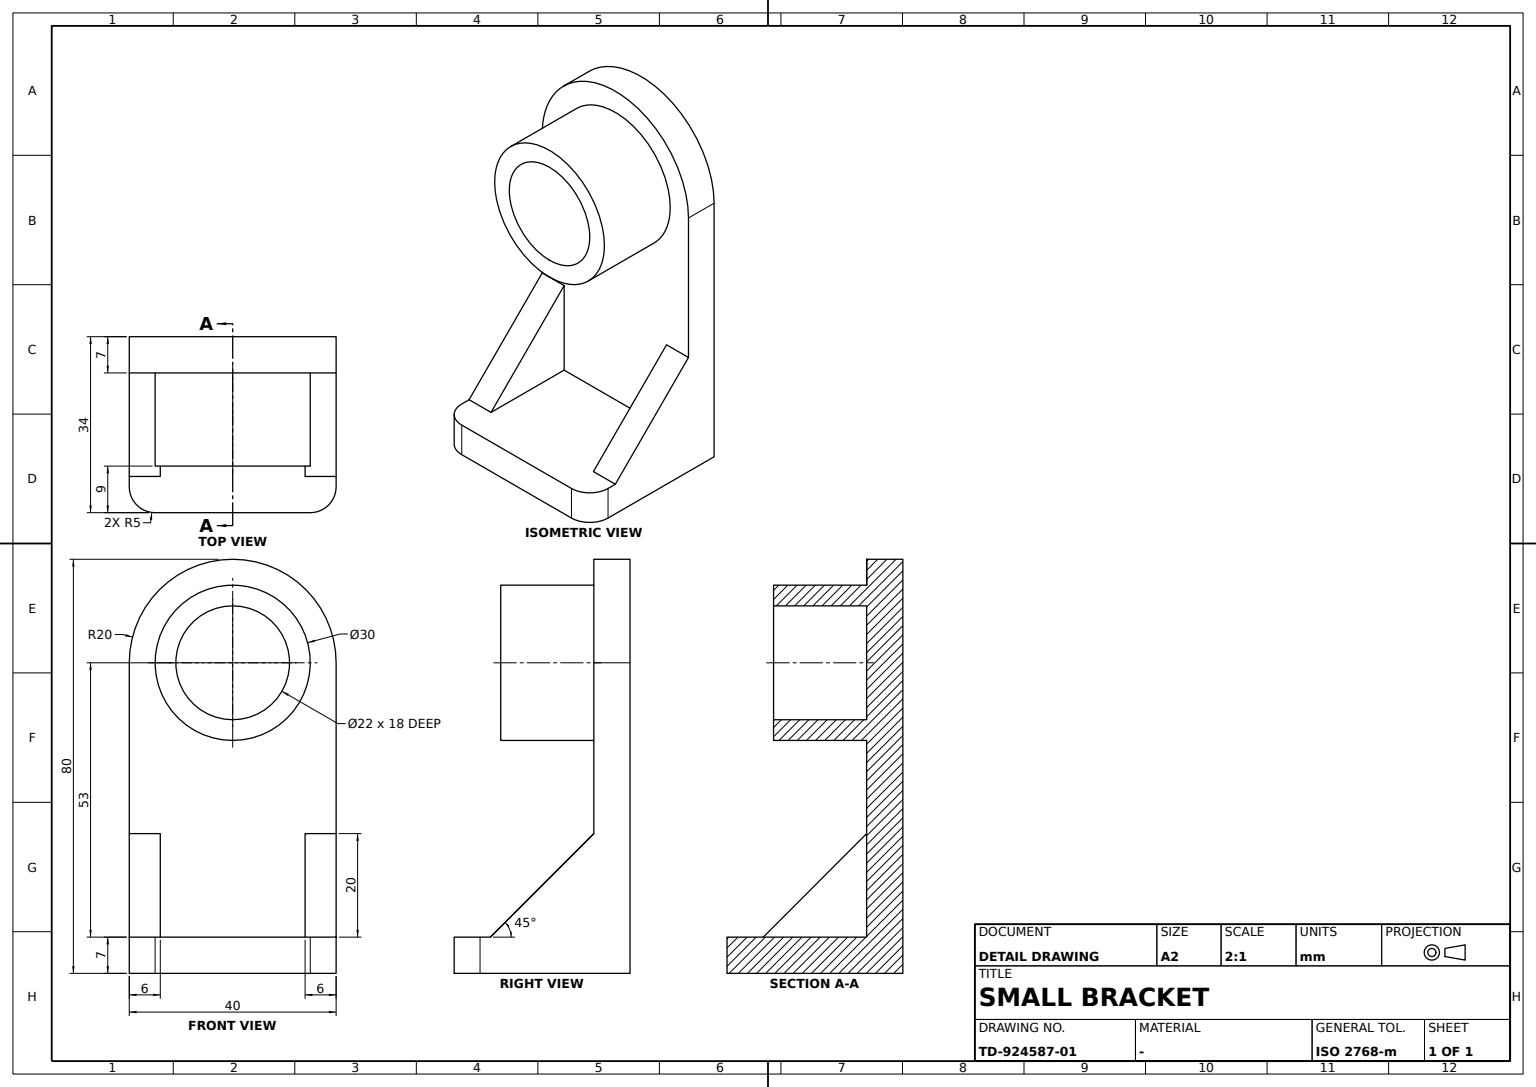
CATIA V5 part; units mm, degrees
sketch "Sketch1" plane through (0, 0, 0) normal (0, 0, 1) x (0, 1, 0)
  line L0 (20, 0) -> (-20, 0)
  line L1 (-20, 0) -> (-20, -34)
  line L2 (-20, -34) -> (20, -34)
  line L3 (20, -34) -> (20, 0)
  dimension "length L1" = 34
  dimension "length L2" = 40
  constraint horizontal L0 x-axis
  constraint horizontal L2 x-axis
  constraint vertical L1 y-axis
  constraint vertical L3 y-axis
  constraint symmetry L1 L3 y-axis
  constraint coincidence L0 x-axis
extrude "Pad1" add sketch "Sketch1" along normal blind 7
fillet "Fillet1" radius 5 2 edges at (34, 20, 3.5) (34, -20, 3.5)
sketch "Sketch2" plane through (0, 0, 0) normal (1, 0, 0) x (0, 1, 0)
  arc A0 (20, 60) -> (-20, 60) centre (0, 60) ccw
  point P0 (0, 60)
  line L0 (-20, 60) -> (-20, 7)
  point P1 (-20, 7)
  line L1 (-15, 7) -> (-20, 7) construction
  point P2 (-20, 7)
  line L2 (-20, 7) -> (20, 7)
  line L3 (20, 7) -> (20, 60)
  dimension "length L0" = 53
  dimension "radius A0" = 20
  dimension "length L3" = 53
  constraint coincidence P0 y-axis
  constraint coincidence P1 L1
  constraint coincidence P2 P1
  constraint vertical L0 y-axis
  constraint tangency L0 A0
  constraint tangency L3 A0
  constraint horizontal L2 x-axis
extrude "Pad2" add sketch "Sketch2" along normal blind 7
sketch "Sketch3" plane through (7, 0, 0) normal (1, 0, 0) x (0, 1, 0)
  circle A0 centre (0, 60) radius 15
  point P0 (0, 60)
  arc A1 (20, 60) -> (-20, 60) centre (0, 60) ccw construction
  circle A2 centre (0, 60) radius 11
  dimension "radius A0" = 15
  dimension "radius A2" = 11
  constraint coincidence P0 y-axis
  constraint concentricity A0 A1
extrude "Pad3" add sketch "Sketch3" along normal blind 18
sketch "Sketch4" plane through (0, 20, 0) normal (0, 1, 0) x (-1, 0, 0)
  line L0 (-27, 7) -> (-7, 7)
  line L1 (-7, 7) -> (-7, 27)
  line L2 (-7, 27) -> (-27, 7)
  line L3 (-34, 7) -> (0, 7) construction
  line L4 (-7, 7) -> (-7, 60) construction
  dimension "length L1" = 20
  dimension "length L0" = 20
  constraint horizontal L0 x-axis
  constraint vertical L1 y-axis
  constraint coincidence L0 L3
  constraint coincidence L1 L4
extrude "Pad4" add sketch "Sketch4" against normal blind 6
mirror "Mirror1" about plane through (0, 0, 0) normal (0, 1, 0) of "Pad4"
